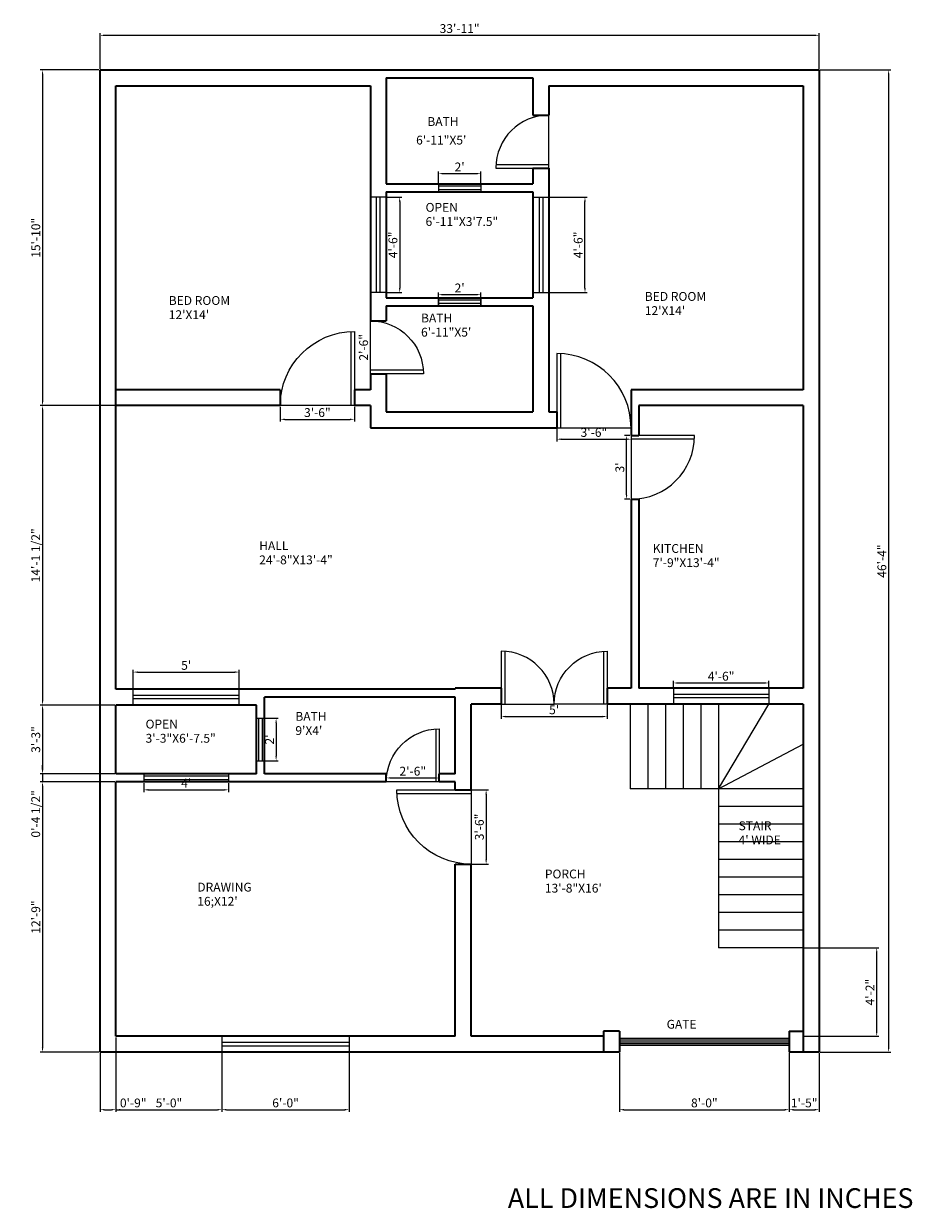
# Model space of a CAD drawing. Units: inches. Extents: x 2169 to 2672, y 1452 to 2123.
import ezdxf

# ---------------------------------------------------------------- set-up
doc = ezdxf.new("R2010")
doc.units = ezdxf.units.IN
for name, color, linetype, lineweight in [('A-ANNO-DIMS', 2, 'Continuous', 18), ('A-ANNO-TEXT', 20, 'Continuous', 18), ('A-AREA-IDEN', 20, 'Continuous', 18), ('A-FLOR-STRS', 200, 'Continuous', 25), ('DOORS', 104, 'Continuous', 25), ('WALL', 200, 'Continuous', 35), ('WINDOWS', 4, 'Continuous', 18)]:
    doc.layers.add(name, color=color, linetype=linetype, lineweight=lineweight)
doc.styles.get("Standard").update_dxf_attribs({"font": 'arial.ttf', "height": 5})
doc.dimstyles.new('ISO-25', dxfattribs={"dimtxt": 5, "dimasz": 2.5, "dimexe": 1.25, "dimexo": 0.625, "dimtad": 1, "dimlunit": 3, "dimtxsty": 'Standard', "dimcen": 2.5, "dimadec": 0, "dimazin": 0, "dimtfac": 1, "dimtmove": 0, "dimatfit": 3, "dimfxl": 1, "dimarcsym": 0})

# ---------------------------------------------------------------- blocks, each defined once
blk = doc.blocks.new('*D1')
at = {"layer": 'A-ANNO-DIMS', "color": 0, "lineweight": -2, "transparency": 16777216}
for p, q in [((2620.28, 2096.79), (2660.2, 2096.79)), ((2658.95, 2094.29), (2658.95, 1543.29)), ((2620.28, 1540.79), (2660.2, 1540.79))]:
    blk.add_line(p, q, dxfattribs=at)
at = {"layer": 'A-ANNO-DIMS', "color": 0, "transparency": 16777216}
for points in [[(2658.53, 2094.29), (2659.36, 2094.29), (2658.95, 2096.79)], [(2658.53, 1543.29), (2659.36, 1543.29), (2658.95, 1540.79)]]:
    blk.add_solid(points, dxfattribs=at)
at = {"layer": 'Defpoints', "color": 0, "transparency": 16777216}
for p in [(2619.65, 2096.79), (2619.65, 1540.79), (2658.95, 1540.79)]:
    blk.add_point(p, dxfattribs=at)
at = {"layer": 'A-ANNO-DIMS', "color": 0, "transparency": 16777216, "insert": (2655.77, 1818.79), "char_height": 5, "attachment_point": 5, "rotation": 90}
blk.add_mtext('46\'-4"', dxfattribs=at)
blk = doc.blocks.new('*D2')
at = {"layer": 'A-ANNO-DIMS', "color": 0, "lineweight": -2, "transparency": 16777216}
for p, q in [((2212.65, 2097.41), (2212.65, 2117.66)), ((2215.15, 2116.41), (2617.15, 2116.41)), ((2619.65, 2097.41), (2619.65, 2117.66))]:
    blk.add_line(p, q, dxfattribs=at)
at = {"layer": 'A-ANNO-DIMS', "color": 0, "transparency": 16777216}
for points in [[(2215.15, 2116.83), (2215.15, 2115.99), (2212.65, 2116.41)], [(2617.15, 2116.83), (2617.15, 2115.99), (2619.65, 2116.41)]]:
    blk.add_solid(points, dxfattribs=at)
at = {"layer": 'Defpoints', "color": 0, "transparency": 16777216}
for p in [(2619.65, 2116.41), (2212.65, 2096.79), (2619.65, 2096.79)]:
    blk.add_point(p, dxfattribs=at)
at = {"layer": 'A-ANNO-DIMS', "color": 0, "transparency": 16777216, "insert": (2416.15, 2119.59), "char_height": 5, "attachment_point": 5}
blk.add_mtext('33\'-11"', dxfattribs=at)
blk = doc.blocks.new('*D3')
at = {"layer": 'A-ANNO-DIMS', "color": 0, "lineweight": -2, "transparency": 16777216}
for p, q in [((2314.65, 1906.16), (2314.65, 1897.78)), ((2356.65, 1906.16), (2356.65, 1897.78)), ((2317.15, 1899.03), (2354.15, 1899.03))]:
    blk.add_line(p, q, dxfattribs=at)
at = {"layer": 'A-ANNO-DIMS', "color": 0, "transparency": 16777216}
for points in [[(2317.15, 1899.45), (2317.15, 1898.62), (2314.65, 1899.03)], [(2354.15, 1899.45), (2354.15, 1898.62), (2356.65, 1899.03)]]:
    blk.add_solid(points, dxfattribs=at)
at = {"layer": 'Defpoints', "color": 0, "transparency": 16777216}
for p in [(2314.65, 1906.79), (2356.65, 1906.79), (2356.65, 1899.03)]:
    blk.add_point(p, dxfattribs=at)
at = {"layer": 'A-ANNO-DIMS', "color": 0, "transparency": 16777216, "insert": (2335.65, 1902.21), "char_height": 5, "attachment_point": 5}
blk.add_mtext('3\'-6"', dxfattribs=at)
blk = doc.blocks.new('*D4')
at = {"layer": 'A-ANNO-DIMS', "color": 0, "lineweight": -2, "transparency": 16777216}
for p, q in [((2365.65, 1927.29), (2365.65, 1952.29)), ((2366.28, 1954.79), (2366.9, 1954.79)), ((2366.28, 1924.79), (2366.9, 1924.79))]:
    blk.add_line(p, q, dxfattribs=at)
at = {"layer": 'A-ANNO-DIMS', "color": 0, "transparency": 16777216}
for points in [[(2365.24, 1952.29), (2366.07, 1952.29), (2365.65, 1954.79)], [(2365.24, 1927.29), (2366.07, 1927.29), (2365.65, 1924.79)]]:
    blk.add_solid(points, dxfattribs=at)
at = {"layer": 'Defpoints', "color": 0, "transparency": 16777216}
for p in [(2365.65, 1954.79), (2365.65, 1954.79), (2365.65, 1924.79)]:
    blk.add_point(p, dxfattribs=at)
at = {"layer": 'A-ANNO-DIMS', "color": 0, "transparency": 16777216, "insert": (2362.48, 1939.79), "char_height": 5, "attachment_point": 5, "rotation": 90}
blk.add_mtext('2\'-6"', dxfattribs=at)
blk = doc.blocks.new('*D5')
at = {"layer": 'A-ANNO-DIMS', "color": 0, "lineweight": -2, "transparency": 16777216}
for p, q in [((2471.15, 1893.66), (2471.15, 1886.54)), ((2513.15, 1893.66), (2513.15, 1886.54)), ((2473.65, 1887.79), (2510.65, 1887.79))]:
    blk.add_line(p, q, dxfattribs=at)
at = {"layer": 'A-ANNO-DIMS', "color": 0, "transparency": 16777216}
for points in [[(2473.65, 1888.21), (2473.65, 1887.37), (2471.15, 1887.79)], [(2510.65, 1888.21), (2510.65, 1887.37), (2513.15, 1887.79)]]:
    blk.add_solid(points, dxfattribs=at)
at = {"layer": 'Defpoints', "color": 0, "transparency": 16777216}
for p in [(2471.15, 1894.29), (2513.15, 1894.29), (2513.15, 1887.79)]:
    blk.add_point(p, dxfattribs=at)
at = {"layer": 'A-ANNO-DIMS', "color": 0, "transparency": 16777216, "insert": (2492.15, 1890.97), "char_height": 5, "attachment_point": 5}
blk.add_mtext('3\'-6"', dxfattribs=at)
blk = doc.blocks.new('*D6')
at = {"layer": 'A-ANNO-DIMS', "color": 0, "lineweight": -2, "transparency": 16777216}
for p, q in [((2512.53, 1889.79), (2509.4, 1889.79)), ((2510.65, 1856.29), (2510.65, 1887.29)), ((2512.53, 1853.79), (2509.4, 1853.79))]:
    blk.add_line(p, q, dxfattribs=at)
at = {"layer": 'A-ANNO-DIMS', "color": 0, "transparency": 16777216}
for points in [[(2510.24, 1887.29), (2511.07, 1887.29), (2510.65, 1889.79)], [(2510.24, 1856.29), (2511.07, 1856.29), (2510.65, 1853.79)]]:
    blk.add_solid(points, dxfattribs=at)
at = {"layer": 'Defpoints', "color": 0, "transparency": 16777216}
for p in [(2510.65, 1889.79), (2513.15, 1889.79), (2513.15, 1853.79)]:
    blk.add_point(p, dxfattribs=at)
at = {"layer": 'A-ANNO-DIMS', "color": 0, "transparency": 16777216, "insert": (2507.47, 1871.79), "char_height": 5, "attachment_point": 5, "rotation": 90}
blk.add_mtext("3'", dxfattribs=at)
blk = doc.blocks.new('*D7')
at = {"layer": 'A-ANNO-DIMS', "color": 0, "lineweight": -2, "transparency": 16777216}
for p, q in [((2439.65, 1737.16), (2439.65, 1729.54)), ((2499.65, 1737.16), (2499.65, 1729.54)), ((2442.15, 1730.79), (2497.15, 1730.79))]:
    blk.add_line(p, q, dxfattribs=at)
at = {"layer": 'A-ANNO-DIMS', "color": 0, "transparency": 16777216}
for points in [[(2442.15, 1731.21), (2442.15, 1730.37), (2439.65, 1730.79)], [(2497.15, 1731.21), (2497.15, 1730.37), (2499.65, 1730.79)]]:
    blk.add_solid(points, dxfattribs=at)
at = {"layer": 'Defpoints', "color": 0, "transparency": 16777216}
for p in [(2439.65, 1737.79), (2499.65, 1737.79), (2499.65, 1730.79)]:
    blk.add_point(p, dxfattribs=at)
at = {"layer": 'A-ANNO-DIMS', "color": 0, "transparency": 16777216, "insert": (2469.65, 1733.96), "char_height": 5, "attachment_point": 5}
blk.add_mtext("5'", dxfattribs=at)
blk = doc.blocks.new('*D8')
at = {"layer": 'A-ANNO-DIMS', "color": 0, "lineweight": -2, "transparency": 16777216}
for p, q in [((2374.65, 1694.54), (2374.65, 1697.29)), ((2404.65, 1694.41), (2404.65, 1697.29)), ((2377.15, 1696.04), (2402.15, 1696.04))]:
    blk.add_line(p, q, dxfattribs=at)
at = {"layer": 'A-ANNO-DIMS', "color": 0, "transparency": 16777216}
for points in [[(2377.15, 1696.46), (2377.15, 1695.62), (2374.65, 1696.04)], [(2402.15, 1696.46), (2402.15, 1695.62), (2404.65, 1696.04)]]:
    blk.add_solid(points, dxfattribs=at)
at = {"layer": 'Defpoints', "color": 0, "transparency": 16777216}
for p in [(2374.65, 1693.92), (2404.65, 1696.04), (2404.65, 1693.79)]:
    blk.add_point(p, dxfattribs=at)
at = {"layer": 'A-ANNO-DIMS', "color": 0, "transparency": 16777216, "insert": (2389.65, 1699.22), "char_height": 5, "attachment_point": 5}
blk.add_mtext('2\'-6"', dxfattribs=at)
blk = doc.blocks.new('*D9')
at = {"layer": 'A-ANNO-DIMS', "color": 0, "lineweight": -2, "transparency": 16777216}
for p, q in [((2423.28, 1689.29), (2432.41, 1689.29)), ((2431.16, 1686.79), (2431.16, 1649.79)), ((2423.28, 1647.29), (2432.41, 1647.29))]:
    blk.add_line(p, q, dxfattribs=at)
at = {"layer": 'A-ANNO-DIMS', "color": 0, "transparency": 16777216}
for points in [[(2430.74, 1686.79), (2431.58, 1686.79), (2431.16, 1689.29)], [(2430.74, 1649.79), (2431.58, 1649.79), (2431.16, 1647.29)]]:
    blk.add_solid(points, dxfattribs=at)
at = {"layer": 'Defpoints', "color": 0, "transparency": 16777216}
for p in [(2422.65, 1689.29), (2422.65, 1647.29), (2431.16, 1647.29)]:
    blk.add_point(p, dxfattribs=at)
at = {"layer": 'A-ANNO-DIMS', "color": 0, "transparency": 16777216, "insert": (2427.98, 1668.29), "char_height": 5, "attachment_point": 5, "rotation": 90}
blk.add_mtext('3\'-6"', dxfattribs=at)
blk = doc.blocks.new('*D10')
at = {"layer": 'A-ANNO-DIMS', "color": 0, "lineweight": -2, "transparency": 16777216}
for p, q in [((2537.15, 1747.41), (2537.15, 1751.04)), ((2591.15, 1747.41), (2591.15, 1751.04)), ((2539.65, 1749.79), (2588.65, 1749.79))]:
    blk.add_line(p, q, dxfattribs=at)
at = {"layer": 'A-ANNO-DIMS', "color": 0, "transparency": 16777216}
for points in [[(2539.65, 1750.2), (2539.65, 1749.37), (2537.15, 1749.79)], [(2588.65, 1750.2), (2588.65, 1749.37), (2591.15, 1749.79)]]:
    blk.add_solid(points, dxfattribs=at)
at = {"layer": 'Defpoints', "color": 0, "transparency": 16777216}
for p in [(2537.15, 1746.79), (2591.15, 1749.79), (2591.15, 1746.79)]:
    blk.add_point(p, dxfattribs=at)
at = {"layer": 'A-ANNO-DIMS', "color": 0, "transparency": 16777216, "insert": (2564.15, 1752.96), "char_height": 5, "attachment_point": 5}
blk.add_mtext('4\'-6"', dxfattribs=at)
blk = doc.blocks.new('*D11')
at = {"layer": 'A-ANNO-DIMS', "color": 0, "lineweight": -2, "transparency": 16777216}
for p, q in [((2231.4, 1746.91), (2231.4, 1757.2)), ((2291.4, 1746.91), (2291.4, 1757.2)), ((2233.9, 1755.95), (2288.9, 1755.95))]:
    blk.add_line(p, q, dxfattribs=at)
at = {"layer": 'A-ANNO-DIMS', "color": 0, "transparency": 16777216}
for points in [[(2233.9, 1756.36), (2233.9, 1755.53), (2231.4, 1755.95)], [(2288.9, 1756.36), (2288.9, 1755.53), (2291.4, 1755.95)]]:
    blk.add_solid(points, dxfattribs=at)
at = {"layer": 'Defpoints', "color": 0, "transparency": 16777216}
for p in [(2291.4, 1755.95), (2231.4, 1746.29), (2291.4, 1746.29)]:
    blk.add_point(p, dxfattribs=at)
at = {"layer": 'A-ANNO-DIMS', "color": 0, "transparency": 16777216, "insert": (2261.4, 1759.11), "char_height": 5, "attachment_point": 5}
blk.add_mtext("5'", dxfattribs=at)
blk = doc.blocks.new('*D12')
at = {"layer": 'A-ANNO-DIMS', "color": 0, "lineweight": -2, "transparency": 16777216}
for p, q in [((2237.4, 1693.16), (2237.4, 1688.06)), ((2285.4, 1693.16), (2285.4, 1688.06)), ((2239.9, 1689.31), (2282.9, 1689.31))]:
    blk.add_line(p, q, dxfattribs=at)
at = {"layer": 'A-ANNO-DIMS', "color": 0, "transparency": 16777216}
for points in [[(2239.9, 1689.73), (2239.9, 1688.89), (2237.4, 1689.31)], [(2282.9, 1689.73), (2282.9, 1688.89), (2285.4, 1689.31)]]:
    blk.add_solid(points, dxfattribs=at)
at = {"layer": 'Defpoints', "color": 0, "transparency": 16777216}
for p in [(2237.4, 1693.79), (2285.4, 1693.79), (2285.4, 1689.31)]:
    blk.add_point(p, dxfattribs=at)
at = {"layer": 'A-ANNO-DIMS', "color": 0, "transparency": 16777216, "insert": (2261.4, 1692.44), "char_height": 5, "attachment_point": 5}
blk.add_mtext("4'", dxfattribs=at)
blk = doc.blocks.new('*D13')
at = {"layer": 'A-ANNO-DIMS', "color": 0, "lineweight": -2, "transparency": 16777216}
for p, q in [((2306.28, 1729.79), (2313.55, 1729.79)), ((2312.3, 1727.29), (2312.3, 1708.29)), ((2306.28, 1705.79), (2313.55, 1705.79))]:
    blk.add_line(p, q, dxfattribs=at)
at = {"layer": 'A-ANNO-DIMS', "color": 0, "transparency": 16777216}
for points in [[(2311.89, 1727.29), (2312.72, 1727.29), (2312.3, 1729.79)], [(2311.89, 1708.29), (2312.72, 1708.29), (2312.3, 1705.79)]]:
    blk.add_solid(points, dxfattribs=at)
at = {"layer": 'Defpoints', "color": 0, "transparency": 16777216}
for p in [(2305.65, 1729.79), (2305.65, 1705.79), (2312.3, 1705.79)]:
    blk.add_point(p, dxfattribs=at)
at = {"layer": 'A-ANNO-DIMS', "color": 0, "transparency": 16777216, "insert": (2309.17, 1717.79), "char_height": 5, "attachment_point": 5, "rotation": 90}
blk.add_mtext("2'", dxfattribs=at)
blk = doc.blocks.new('*D14')
at = {"layer": 'A-ANNO-DIMS', "color": 0, "lineweight": -2, "transparency": 16777216}
for p, q in [((2404.15, 2032.91), (2404.15, 2039.36)), ((2428.15, 2032.91), (2428.15, 2039.36)), ((2406.65, 2038.11), (2425.65, 2038.11))]:
    blk.add_line(p, q, dxfattribs=at)
at = {"layer": 'A-ANNO-DIMS', "color": 0, "transparency": 16777216}
for points in [[(2406.65, 2038.53), (2406.65, 2037.69), (2404.15, 2038.11)], [(2425.65, 2038.53), (2425.65, 2037.69), (2428.15, 2038.11)]]:
    blk.add_solid(points, dxfattribs=at)
at = {"layer": 'Defpoints', "color": 0, "transparency": 16777216}
for p in [(2404.15, 2032.29), (2428.15, 2038.11), (2428.15, 2032.29)]:
    blk.add_point(p, dxfattribs=at)
at = {"layer": 'A-ANNO-DIMS', "color": 0, "transparency": 16777216, "insert": (2416.15, 2041.25), "char_height": 5, "attachment_point": 5}
blk.add_mtext("2'", dxfattribs=at)
blk = doc.blocks.new('*D15')
at = {"layer": 'A-ANNO-DIMS', "color": 0, "lineweight": -2, "transparency": 16777216}
for p, q in [((2375.28, 2024.79), (2383.5, 2024.79)), ((2382.25, 2022.29), (2382.25, 1973.29)), ((2375.28, 1970.79), (2383.5, 1970.79))]:
    blk.add_line(p, q, dxfattribs=at)
at = {"layer": 'A-ANNO-DIMS', "color": 0, "transparency": 16777216}
for points in [[(2381.83, 2022.29), (2382.66, 2022.29), (2382.25, 2024.79)], [(2381.83, 1973.29), (2382.66, 1973.29), (2382.25, 1970.79)]]:
    blk.add_solid(points, dxfattribs=at)
at = {"layer": 'Defpoints', "color": 0, "transparency": 16777216}
for p in [(2374.65, 2024.79), (2374.65, 1970.79), (2382.25, 1970.79)]:
    blk.add_point(p, dxfattribs=at)
at = {"layer": 'A-ANNO-DIMS', "color": 0, "transparency": 16777216, "insert": (2379.07, 1997.79), "char_height": 5, "attachment_point": 5, "rotation": 90}
blk.add_mtext('4\'-6"', dxfattribs=at)
blk = doc.blocks.new('*D16')
at = {"layer": 'A-ANNO-DIMS', "color": 0, "lineweight": -2, "transparency": 16777216}
for p, q in [((2467.28, 2024.79), (2488.36, 2024.79)), ((2487.11, 1973.29), (2487.11, 2022.29)), ((2467.28, 1970.79), (2488.36, 1970.79))]:
    blk.add_line(p, q, dxfattribs=at)
at = {"layer": 'A-ANNO-DIMS', "color": 0, "transparency": 16777216}
for points in [[(2486.69, 2022.29), (2487.52, 2022.29), (2487.11, 2024.79)], [(2486.69, 1973.29), (2487.52, 1973.29), (2487.11, 1970.79)]]:
    blk.add_solid(points, dxfattribs=at)
at = {"layer": 'Defpoints', "color": 0, "transparency": 16777216}
for p in [(2466.65, 2024.79), (2487.11, 2024.79), (2466.65, 1970.79)]:
    blk.add_point(p, dxfattribs=at)
at = {"layer": 'A-ANNO-DIMS', "color": 0, "transparency": 16777216, "insert": (2483.93, 1997.79), "char_height": 5, "attachment_point": 5, "rotation": 90}
blk.add_mtext('4\'-6"', dxfattribs=at)
blk = doc.blocks.new('*D17')
at = {"layer": 'A-ANNO-DIMS', "color": 0, "lineweight": -2, "transparency": 16777216}
for p, q in [((2404.15, 1963.91), (2404.15, 1970.86)), ((2406.65, 1969.61), (2425.65, 1969.61)), ((2428.15, 1963.91), (2428.15, 1970.86))]:
    blk.add_line(p, q, dxfattribs=at)
at = {"layer": 'A-ANNO-DIMS', "color": 0, "transparency": 16777216}
for points in [[(2406.65, 1970.03), (2406.65, 1969.19), (2404.15, 1969.61)], [(2425.65, 1970.03), (2425.65, 1969.19), (2428.15, 1969.61)]]:
    blk.add_solid(points, dxfattribs=at)
at = {"layer": 'Defpoints', "color": 0, "transparency": 16777216}
for p in [(2428.15, 1969.61), (2404.15, 1963.29), (2428.15, 1963.29)]:
    blk.add_point(p, dxfattribs=at)
at = {"layer": 'A-ANNO-DIMS', "color": 0, "transparency": 16777216, "insert": (2416.15, 1972.74), "char_height": 5, "attachment_point": 5}
blk.add_mtext("2'", dxfattribs=at)
blk = doc.blocks.new('DOOR-SWING-30IN')
for p, q in [((0, 30), (0, 0)), ((2, 29.93), (2, 0)), ((0, 0), (30, 0))]:
    blk.add_line(p, q)
blk.add_arc((0, 0), 30, 0, 90)
blk = doc.blocks.new('DOOR-SWING-42IN')
for p, q in [((0, 42), (0, 0)), ((2, 41.95), (2, 0)), ((0, 0), (42, 0))]:
    blk.add_line(p, q)
blk.add_arc((0, 0), 42, 0, 90)
blk = doc.blocks.new('WIN-54IN-9IN-WALL')
for p, q in [((0, 9), (0, 0)), ((0, 9), (54, 9)), ((54, 9), (54, 0)), ((54, 5.5), (0, 5.5)), ((54, 3.5), (0, 3.5)), ((0, 0), (54, 0))]:
    blk.add_line(p, q)
blk = doc.blocks.new('WIN-24IN-4_5IN-WALL')
for p, q in [((0, 24), (4.5, 24)), ((0, 24), (0, 0)), ((1.25, 24), (1.25, 0)), ((3.25, 24), (3.25, 0)), ((4.5, 24), (4.5, 0)), ((0, 0), (4.5, 0))]:
    blk.add_line(p, q)
blk = doc.blocks.new('*D22')
at = {"layer": 'A-ANNO-DIMS', "color": 0, "lineweight": -2, "transparency": 16777216}
for p, q in [((2221.65, 1549.16), (2221.65, 1506.99)), ((2212.65, 1540.16), (2212.65, 1506.99)), ((2215.15, 1508.24), (2219.15, 1508.24)), ((2221.65, 1508.24), (2238.7, 1508.24))]:
    blk.add_line(p, q, dxfattribs=at)
at = {"layer": 'A-ANNO-DIMS', "color": 0, "transparency": 16777216}
for points in [[(2215.15, 1508.66), (2215.15, 1507.82), (2212.65, 1508.24)], [(2219.15, 1508.66), (2219.15, 1507.82), (2221.65, 1508.24)]]:
    blk.add_solid(points, dxfattribs=at)
at = {"layer": 'Defpoints', "color": 0, "transparency": 16777216}
for p in [(2221.65, 1549.79), (2212.65, 1540.79), (2221.65, 1508.24)]:
    blk.add_point(p, dxfattribs=at)
at = {"layer": 'A-ANNO-DIMS', "color": 0, "transparency": 16777216, "insert": (2231.42, 1511.42), "char_height": 5, "attachment_point": 5}
blk.add_mtext('0\'-9"', dxfattribs=at)
blk = doc.blocks.new('*D23')
at = {"layer": 'A-ANNO-DIMS', "color": 0, "lineweight": -2, "transparency": 16777216}
for p, q in [((2221.65, 1549.16), (2221.65, 1506.99)), ((2281.65, 1540.16), (2281.65, 1506.99)), ((2224.15, 1508.24), (2279.15, 1508.24))]:
    blk.add_line(p, q, dxfattribs=at)
at = {"layer": 'A-ANNO-DIMS', "color": 0, "transparency": 16777216}
for points in [[(2224.15, 1508.66), (2224.15, 1507.82), (2221.65, 1508.24)], [(2279.15, 1508.66), (2279.15, 1507.82), (2281.65, 1508.24)]]:
    blk.add_solid(points, dxfattribs=at)
at = {"layer": 'Defpoints', "color": 0, "transparency": 16777216}
for p in [(2221.65, 1549.79), (2281.65, 1540.79), (2281.65, 1508.24)]:
    blk.add_point(p, dxfattribs=at)
at = {"layer": 'A-ANNO-DIMS', "color": 0, "transparency": 16777216, "insert": (2251.65, 1511.42), "char_height": 5, "attachment_point": 5}
blk.add_mtext('5\'-0"', dxfattribs=at)
blk = doc.blocks.new('*D24')
at = {"layer": 'A-ANNO-DIMS', "color": 0, "lineweight": -2, "transparency": 16777216}
for p, q in [((2281.65, 1540.16), (2281.65, 1506.99)), ((2353.65, 1540.16), (2353.65, 1506.99)), ((2284.15, 1508.24), (2351.15, 1508.24))]:
    blk.add_line(p, q, dxfattribs=at)
at = {"layer": 'A-ANNO-DIMS', "color": 0, "transparency": 16777216}
for points in [[(2284.15, 1508.66), (2284.15, 1507.82), (2281.65, 1508.24)], [(2351.15, 1508.66), (2351.15, 1507.82), (2353.65, 1508.24)]]:
    blk.add_solid(points, dxfattribs=at)
at = {"layer": 'Defpoints', "color": 0, "transparency": 16777216}
for p in [(2281.65, 1540.79), (2353.65, 1540.79), (2353.65, 1508.24)]:
    blk.add_point(p, dxfattribs=at)
at = {"layer": 'A-ANNO-DIMS', "color": 0, "transparency": 16777216, "insert": (2317.65, 1511.42), "char_height": 5, "attachment_point": 5}
blk.add_mtext('6\'-0"', dxfattribs=at)
blk = doc.blocks.new('*D25')
at = {"layer": 'A-ANNO-DIMS', "color": 0, "lineweight": -2, "transparency": 16777216}
for p, q in [((2506.65, 1540.16), (2506.65, 1506.99)), ((2602.65, 1540.16), (2602.65, 1506.99)), ((2509.15, 1508.24), (2600.15, 1508.24))]:
    blk.add_line(p, q, dxfattribs=at)
at = {"layer": 'A-ANNO-DIMS', "color": 0, "transparency": 16777216}
for points in [[(2509.15, 1508.66), (2509.15, 1507.82), (2506.65, 1508.24)], [(2600.15, 1508.66), (2600.15, 1507.82), (2602.65, 1508.24)]]:
    blk.add_solid(points, dxfattribs=at)
at = {"layer": 'Defpoints', "color": 0, "transparency": 16777216}
for p in [(2506.65, 1540.79), (2602.65, 1540.79), (2602.65, 1508.24)]:
    blk.add_point(p, dxfattribs=at)
at = {"layer": 'A-ANNO-DIMS', "color": 0, "transparency": 16777216, "insert": (2554.65, 1511.42), "char_height": 5, "attachment_point": 5}
blk.add_mtext('8\'-0"', dxfattribs=at)
blk = doc.blocks.new('*D26')
at = {"layer": 'A-ANNO-DIMS', "color": 0, "lineweight": -2, "transparency": 16777216}
for p, q in [((2602.65, 1540.16), (2602.65, 1506.99)), ((2619.65, 1540.16), (2619.65, 1506.99)), ((2605.15, 1508.24), (2617.15, 1508.24))]:
    blk.add_line(p, q, dxfattribs=at)
at = {"layer": 'A-ANNO-DIMS', "color": 0, "transparency": 16777216}
for points in [[(2605.15, 1508.66), (2605.15, 1507.82), (2602.65, 1508.24)], [(2617.15, 1508.66), (2617.15, 1507.82), (2619.65, 1508.24)]]:
    blk.add_solid(points, dxfattribs=at)
at = {"layer": 'Defpoints', "color": 0, "transparency": 16777216}
for p in [(2602.65, 1540.79), (2619.65, 1540.79), (2619.65, 1508.24)]:
    blk.add_point(p, dxfattribs=at)
at = {"layer": 'A-ANNO-DIMS', "color": 0, "transparency": 16777216, "insert": (2611.15, 1511.42), "char_height": 5, "attachment_point": 5}
blk.add_mtext('1\'-5"', dxfattribs=at)
blk = doc.blocks.new('*D27')
at = {"layer": 'A-ANNO-DIMS', "color": 0, "lineweight": -2, "transparency": 16777216}
for p, q in [((2611.28, 1599.79), (2653.45, 1599.79)), ((2652.2, 1552.29), (2652.2, 1597.29)), ((2611.28, 1549.79), (2653.45, 1549.79))]:
    blk.add_line(p, q, dxfattribs=at)
at = {"layer": 'A-ANNO-DIMS', "color": 0, "transparency": 16777216}
for points in [[(2651.79, 1597.29), (2652.62, 1597.29), (2652.2, 1599.79)], [(2651.79, 1552.29), (2652.62, 1552.29), (2652.2, 1549.79)]]:
    blk.add_solid(points, dxfattribs=at)
at = {"layer": 'Defpoints', "color": 0, "transparency": 16777216}
for p in [(2610.65, 1599.79), (2652.2, 1599.79), (2610.65, 1549.79)]:
    blk.add_point(p, dxfattribs=at)
at = {"layer": 'A-ANNO-DIMS', "color": 0, "transparency": 16777216, "insert": (2649.07, 1574.79), "char_height": 5, "attachment_point": 5, "rotation": 90}
blk.add_mtext('4\'-2"', dxfattribs=at)
blk = doc.blocks.new('*D28')
at = {"layer": 'A-ANNO-DIMS', "color": 0, "lineweight": -2, "transparency": 16777216}
for p, q in [((2212.03, 2096.79), (2178.85, 2096.79)), ((2180.1, 2094.29), (2180.1, 1909.29)), ((2221.03, 1906.79), (2178.85, 1906.79))]:
    blk.add_line(p, q, dxfattribs=at)
at = {"layer": 'A-ANNO-DIMS', "color": 0, "transparency": 16777216}
for points in [[(2179.69, 2094.29), (2180.52, 2094.29), (2180.1, 2096.79)], [(2179.69, 1909.29), (2180.52, 1909.29), (2180.1, 1906.79)]]:
    blk.add_solid(points, dxfattribs=at)
at = {"layer": 'Defpoints', "color": 0, "transparency": 16777216}
for p in [(2212.65, 2096.79), (2180.1, 1906.79), (2221.65, 1906.79)]:
    blk.add_point(p, dxfattribs=at)
at = {"layer": 'A-ANNO-DIMS', "color": 0, "transparency": 16777216, "insert": (2176.93, 2001.79), "char_height": 5, "attachment_point": 5, "rotation": 90}
blk.add_mtext('15\'-10"', dxfattribs=at)
blk = doc.blocks.new('*D29')
at = {"layer": 'A-ANNO-DIMS', "color": 0, "lineweight": -2, "transparency": 16777216}
for p, q in [((2221.03, 1906.79), (2178.85, 1906.79)), ((2180.1, 1904.29), (2180.1, 1739.79)), ((2221.03, 1737.29), (2178.85, 1737.29))]:
    blk.add_line(p, q, dxfattribs=at)
at = {"layer": 'A-ANNO-DIMS', "color": 0, "transparency": 16777216}
for points in [[(2179.69, 1904.29), (2180.52, 1904.29), (2180.1, 1906.79)], [(2179.69, 1739.79), (2180.52, 1739.79), (2180.1, 1737.29)]]:
    blk.add_solid(points, dxfattribs=at)
at = {"layer": 'Defpoints', "color": 0, "transparency": 16777216}
for p in [(2221.65, 1906.79), (2180.1, 1737.29), (2221.65, 1737.29)]:
    blk.add_point(p, dxfattribs=at)
at = {"layer": 'A-ANNO-DIMS', "color": 0, "transparency": 16777216, "insert": (2176.89, 1822.04), "char_height": 5, "attachment_point": 5, "rotation": 90}
blk.add_mtext('14\'-1 1/2"', dxfattribs=at)
blk = doc.blocks.new('*D30')
at = {"layer": 'A-ANNO-DIMS', "color": 0, "lineweight": -2, "transparency": 16777216}
for p, q in [((2221.03, 1737.29), (2178.85, 1737.29)), ((2180.1, 1734.79), (2180.1, 1700.79)), ((2221.03, 1698.29), (2178.85, 1698.29))]:
    blk.add_line(p, q, dxfattribs=at)
at = {"layer": 'A-ANNO-DIMS', "color": 0, "transparency": 16777216}
for points in [[(2179.69, 1734.79), (2180.52, 1734.79), (2180.1, 1737.29)], [(2179.69, 1700.79), (2180.52, 1700.79), (2180.1, 1698.29)]]:
    blk.add_solid(points, dxfattribs=at)
at = {"layer": 'Defpoints', "color": 0, "transparency": 16777216}
for p in [(2221.65, 1737.29), (2180.1, 1698.29), (2221.65, 1698.29)]:
    blk.add_point(p, dxfattribs=at)
at = {"layer": 'A-ANNO-DIMS', "color": 0, "transparency": 16777216, "insert": (2176.92, 1717.79), "char_height": 5, "attachment_point": 5, "rotation": 90}
blk.add_mtext('3\'-3"', dxfattribs=at)
blk = doc.blocks.new('*D31')
at = {"layer": 'A-ANNO-DIMS', "color": 0, "lineweight": -2, "transparency": 16777216}
for p, q in [((2180.1, 1700.79), (2180.1, 1703.29)), ((2221.03, 1698.29), (2178.85, 1698.29)), ((2180.1, 1698.29), (2180.1, 1693.79)), ((2221.03, 1693.79), (2178.85, 1693.79)), ((2180.1, 1691.29), (2180.1, 1662.6))]:
    blk.add_line(p, q, dxfattribs=at)
at = {"layer": 'A-ANNO-DIMS', "color": 0, "transparency": 16777216}
for points in [[(2179.69, 1700.79), (2180.52, 1700.79), (2180.1, 1698.29)], [(2179.69, 1691.29), (2180.52, 1691.29), (2180.1, 1693.79)]]:
    blk.add_solid(points, dxfattribs=at)
at = {"layer": 'Defpoints', "color": 0, "transparency": 16777216}
for p in [(2221.65, 1698.29), (2180.1, 1693.79), (2221.65, 1693.79)]:
    blk.add_point(p, dxfattribs=at)
at = {"layer": 'A-ANNO-DIMS', "color": 0, "transparency": 16777216, "insert": (2176.89, 1675.69), "char_height": 5, "attachment_point": 5, "rotation": 90}
blk.add_mtext('0\'-4 1/2"', dxfattribs=at)
blk = doc.blocks.new('*D32')
at = {"layer": 'A-ANNO-DIMS', "color": 0, "lineweight": -2, "transparency": 16777216}
for p, q in [((2221.03, 1693.79), (2178.85, 1693.79)), ((2180.1, 1691.29), (2180.1, 1543.29)), ((2212.03, 1540.79), (2178.85, 1540.79))]:
    blk.add_line(p, q, dxfattribs=at)
at = {"layer": 'A-ANNO-DIMS', "color": 0, "transparency": 16777216}
for points in [[(2179.69, 1691.29), (2180.52, 1691.29), (2180.1, 1693.79)], [(2179.69, 1543.29), (2180.52, 1543.29), (2180.1, 1540.79)]]:
    blk.add_solid(points, dxfattribs=at)
at = {"layer": 'Defpoints', "color": 0, "transparency": 16777216}
for p in [(2221.65, 1693.79), (2180.1, 1540.79), (2212.65, 1540.79)]:
    blk.add_point(p, dxfattribs=at)
at = {"layer": 'A-ANNO-DIMS', "color": 0, "transparency": 16777216, "insert": (2176.93, 1617.29), "char_height": 5, "attachment_point": 5, "rotation": 90}
blk.add_mtext('12\'-9"', dxfattribs=at)

msp = doc.modelspace()

# ---------------------------------------------------------------- linework, layer by layer
at = {"layer": 'A-FLOR-STRS'}
for p, q in [((2512.654, 1737.789), (2512.654, 1689.789)), ((2522.654, 1737.789), (2522.654, 1689.789)), ((2532.654, 1737.789), (2532.654, 1689.789)), ((2542.654, 1737.789), (2542.654, 1689.789)), ((2552.654, 1737.789), (2552.654, 1689.789)), ((2562.654, 1737.789), (2562.654, 1599.789)), ((2562.654, 1689.789), (2591.154, 1737.789)), ((2562.654, 1689.789), (2610.654, 1715.216)), ((2610.654, 1689.789), (2512.654, 1689.789)), ((2610.654, 1679.789), (2562.654, 1679.789)), ((2610.654, 1669.789), (2562.654, 1669.789)), ((2610.654, 1659.789), (2562.654, 1659.789)), ((2610.654, 1649.789), (2562.654, 1649.789)), ((2610.654, 1639.789), (2562.654, 1639.789)), ((2610.654, 1629.789), (2562.654, 1629.789)), ((2610.654, 1619.789), (2562.654, 1619.789)), ((2610.654, 1609.789), (2562.654, 1609.789)), ((2610.654, 1599.789), (2562.654, 1599.789))]:
    msp.add_line(p, q, dxfattribs=at)
at = {"layer": 'DOORS'}
for p, q in [((2549.154, 1889.789), (2513.154, 1889.789)), ((2513.154, 1889.789), (2513.154, 1853.789)), ((2549.098, 1887.789), (2513.154, 1887.789)), ((2506.654, 1548.708), (2602.654, 1548.708)), ((2506.654, 1547.708), (2602.654, 1547.708)), ((2506.654, 1546.708), (2602.654, 1546.708)), ((2506.654, 1545.708), (2602.654, 1545.708)), ((2506.654, 1544.708), (2602.654, 1544.708))]:
    msp.add_line(p, q, dxfattribs=at)
msp.add_arc((2513.154, 1889.789), 36, 270, 0, dxfattribs=at)
at = {"layer": 'WALL'}
for p, q in [((2212.654, 2096.789), (2619.654, 2096.789)), ((2212.654, 1540.789), (2212.654, 2096.789)), ((2374.654, 2092.289), (2374.654, 2032.289)), ((2374.654, 2092.289), (2457.654, 2092.289)), ((2457.654, 2092.289), (2457.654, 2071.289)), ((2619.654, 2096.789), (2619.654, 1540.789)), ((2221.654, 2087.789), (2365.654, 2087.789)), ((2221.654, 1746.289), (2221.654, 2087.789)), ((2365.654, 2087.789), (2365.654, 1954.789)), ((2466.654, 2087.789), (2466.654, 2071.289)), ((2466.654, 2087.789), (2610.654, 2087.789)), ((2610.654, 2087.789), (2610.654, 1915.789)), ((2457.654, 2071.289), (2466.654, 2071.289)), ((2457.654, 2041.289), (2466.654, 2041.289)), ((2457.654, 2041.289), (2457.654, 2032.289)), ((2466.654, 2041.289), (2466.654, 1903.289)), ((2374.654, 2032.289), (2457.654, 2032.289)), ((2374.654, 2027.789), (2457.654, 2027.789)), ((2374.654, 2027.789), (2374.654, 1967.789)), ((2457.654, 2027.789), (2457.654, 1967.789)), ((2374.654, 1967.789), (2457.654, 1967.789)), ((2374.654, 1963.289), (2457.654, 1963.289)), ((2374.654, 1963.289), (2374.654, 1954.789)), ((2457.654, 1963.289), (2457.654, 1903.289)), ((2365.654, 1954.789), (2374.654, 1954.789)), ((2365.654, 1924.789), (2374.654, 1924.789)), ((2365.654, 1924.789), (2365.654, 1915.789)), ((2374.654, 1924.789), (2374.654, 1903.289)), ((2314.654, 1915.789), (2221.654, 1915.789)), ((2314.654, 1915.789), (2314.654, 1906.789)), ((2365.654, 1915.789), (2356.654, 1915.789)), ((2356.654, 1915.789), (2356.654, 1906.789)), ((2610.654, 1915.789), (2513.154, 1915.789)), ((2513.154, 1915.789), (2513.154, 1889.789)), ((2314.654, 1906.789), (2221.654, 1906.789)), ((2365.654, 1906.789), (2356.654, 1906.789)), ((2365.654, 1906.789), (2365.654, 1894.289)), ((2610.654, 1906.789), (2517.654, 1906.789)), ((2517.654, 1906.789), (2517.654, 1889.789)), ((2610.654, 1906.789), (2610.654, 1746.789)), ((2374.654, 1903.289), (2457.654, 1903.289)), ((2466.654, 1903.289), (2471.154, 1903.289)), ((2471.154, 1903.289), (2471.154, 1894.289)), ((2365.654, 1894.289), (2471.154, 1894.289)), ((2513.154, 1889.789), (2517.654, 1889.789)), ((2513.154, 1853.789), (2517.654, 1853.789)), ((2513.154, 1853.789), (2513.154, 1746.789)), ((2517.654, 1853.789), (2517.654, 1746.789)), ((2413.607, 1746.289), (2221.654, 1746.289)), ((2413.607, 1746.289), (2221.654, 1746.289)), ((2413.607, 1746.289), (2413.607, 1746.789)), ((2439.654, 1746.789), (2413.607, 1746.789)), ((2439.654, 1746.789), (2439.654, 1737.789)), ((2513.154, 1746.789), (2499.654, 1746.789)), ((2499.654, 1746.789), (2499.654, 1737.789)), ((2610.654, 1746.789), (2517.654, 1746.789)), ((2301.154, 1737.289), (2221.654, 1737.289)), ((2221.654, 1698.289), (2221.654, 1737.289)), ((2301.154, 1698.289), (2301.154, 1737.289)), ((2413.607, 1741.789), (2305.654, 1741.789)), ((2305.654, 1698.289), (2305.654, 1741.789)), ((2413.607, 1698.289), (2413.607, 1741.789)), ((2439.654, 1737.789), (2422.654, 1737.789)), ((2422.654, 1689.289), (2422.654, 1737.789)), ((2610.654, 1737.789), (2499.654, 1737.789)), ((2610.654, 1737.789), (2610.654, 1549.789)), ((2301.154, 1698.289), (2221.654, 1698.289)), ((2374.609, 1698.289), (2305.654, 1698.289)), ((2374.656, 1693.789), (2374.609, 1698.289)), ((2413.607, 1698.289), (2404.607, 1698.289)), ((2404.654, 1693.789), (2404.607, 1698.289)), ((2221.654, 1549.789), (2221.654, 1693.789)), ((2374.656, 1693.789), (2221.654, 1693.789)), ((2413.654, 1693.789), (2404.654, 1693.789)), ((2413.654, 1689.289), (2413.654, 1693.789)), ((2413.654, 1689.289), (2422.654, 1689.289)), ((2413.654, 1549.789), (2413.654, 1647.289)), ((2413.654, 1647.289), (2422.654, 1647.289)), ((2422.654, 1549.789), (2422.654, 1647.289)), ((2413.654, 1549.789), (2221.654, 1549.789)), ((2497.654, 1549.789), (2422.654, 1549.789)), ((2497.654, 1552.628), (2497.654, 1540.789)), ((2506.654, 1552.628), (2497.654, 1552.628)), ((2506.654, 1552.628), (2506.654, 1540.789)), ((2602.654, 1552.628), (2602.654, 1540.789)), ((2602.654, 1552.628), (2610.654, 1552.628)), ((2610.654, 1549.789), (2610.654, 1540.789)), ((2506.654, 1540.789), (2212.654, 1540.789)), ((2619.654, 1540.789), (2602.654, 1540.789))]:
    msp.add_line(p, q, dxfattribs=at)
at = {"layer": 'WINDOWS'}
for p, q in [((2231.404, 1737.289), (2231.404, 1746.289)), ((2291.404, 1737.289), (2291.404, 1746.289)), ((2291.404, 1742.789), (2231.404, 1742.789)), ((2291.404, 1740.789), (2231.404, 1740.789)), ((2237.404, 1698.289), (2237.404, 1693.789)), ((2285.404, 1698.289), (2237.404, 1698.289)), ((2285.404, 1697.039), (2237.404, 1697.039)), ((2285.404, 1698.289), (2285.404, 1693.789)), ((2285.404, 1695.039), (2237.404, 1695.039)), ((2237.404, 1693.789), (2285.404, 1693.789)), ((2281.654, 1549.789), (2281.654, 1540.789)), ((2281.654, 1549.789), (2353.654, 1549.789)), ((2353.654, 1549.789), (2353.654, 1540.789)), ((2353.654, 1546.289), (2281.654, 1546.289)), ((2353.654, 1544.289), (2281.654, 1544.289)), ((2281.654, 1540.789), (2353.654, 1540.789))]:
    msp.add_line(p, q, dxfattribs=at)

# ---------------------------------------------------------------- block references
at = {"layer": 'DOORS', "rotation": 89.99999999999774}
msp.add_blockref('DOOR-SWING-30IN', (2466.654, 2041.289), dxfattribs=at)
at = {"layer": 'DOORS', "extrusion": (0, 0, -1), "zscale": -1}
for name, p, rotation in [('DOOR-SWING-30IN', (-2365.654, 1924.789), 90.00000000000047), ('DOOR-SWING-42IN', (-2422.654, 1689.289), 269.9999999999988)]:
    msp.add_blockref(name, p, dxfattribs=dict(at, rotation=rotation))
for name, p in [('DOOR-SWING-42IN', (-2356.654, 1906.789)), ('DOOR-SWING-30IN', (-2499.654, 1737.789)), ('DOOR-SWING-30IN', (-2404.654, 1693.789))]:
    msp.add_blockref(name, p, dxfattribs=at)
at = {"layer": 'DOORS'}
for name, p in [('DOOR-SWING-42IN', (2471.154, 1894.289)), ('DOOR-SWING-30IN', (2439.654, 1737.789))]:
    msp.add_blockref(name, p, dxfattribs=at)
at = {"layer": 'WINDOWS'}
for name, p, rotation in [('WIN-24IN-4_5IN-WALL', (2404.154, 2032.289), 270.0000000000075), ('WIN-54IN-9IN-WALL', (2365.654, 2024.789), 269.9999999999996), ('WIN-54IN-9IN-WALL', (2466.654, 1970.789), 90.00000000000291), ('WIN-24IN-4_5IN-WALL', (2404.154, 1967.789), 270.0000000000075)]:
    msp.add_blockref(name, p, dxfattribs=dict(at, rotation=rotation))
for name, p in [('WIN-54IN-9IN-WALL', (2537.154, 1737.789)), ('WIN-24IN-4_5IN-WALL', (2301.154, 1705.789))]:
    msp.add_blockref(name, p, dxfattribs=at)

# ---------------------------------------------------------------- texts
at = {"layer": 'A-ANNO-TEXT'}
for s, height, p in [('STAIR', 5, (2574.039, 1666.458)), ("4' WIDE", 5, (2574.039, 1658.426)), ('GATE', 5, (2533.316, 1554.09)), ('ALL DIMENSIONS ARE IN INCHES', 11.17446, (2443.42, 1452.615))]:
    msp.add_text(s, height=height, dxfattribs=at).set_placement(p)
at = {"layer": 'A-AREA-IDEN'}
for s, p in [('BATH', (2397.889, 2065.104)), ('6\'-11"X5\'', (2391.525, 2054.592)), ('OPEN', (2396.869, 2016.521)), ('6\'-11"X3\'7.5"', (2396.869, 2008.489)), ('BED ROOM', (2251.523, 1963.798)), ('BED ROOM', (2520.955, 1966.109)), ("12'X14'", (2251.523, 1955.766)), ('BATH', (2394.319, 1953.889)), ("12'X14'", (2520.955, 1958.077)), ('6\'-11"X5\'', (2394.319, 1945.857)), ('HALL', (2302.719, 1825.006)), ('KITCHEN', (2525.462, 1823.433)), ('24\'-8"X13\'-4"', (2302.719, 1816.974)), ('7\'-9"X13\'-4"', (2525.462, 1815.401)), ('BATH', (2323.188, 1728.374)), ('OPEN', (2238.406, 1724.014)), ("9'X4'", (2323.188, 1720.342)), ('3\'-3"X6\'-7.5"', (2238.406, 1715.982)), ('PORCH', (2464.393, 1639.17)), ('DRAWING', (2267.695, 1631.734)), ('13\'-8"X16\'', (2464.393, 1631.138)), ("16;X12'", (2267.695, 1623.702))]:
    msp.add_text(s, height=5, dxfattribs=at).set_placement(p)

# ---------------------------------------------------------------- dimensions: what is measured, and where the dimension line sits
at = {"layer": 'A-ANNO-DIMS'}
for base, p1, p2, override, picture, middle in [((2619.654, 2116.409), (2212.654, 2096.789), (2619.654, 2096.789), {"dimclrd": 0, "dimclre": 0, "dimclrt": 0}, '*D2', (2416.154, 2119.589)), ((2428.154, 2038.11), (2404.154, 2032.289), (2428.154, 2032.289), {"dimclrd": 0, "dimclre": 0, "dimclrt": 0}, '*D14', (2416.154, 2041.245)), ((2428.154, 1969.609), (2404.154, 1963.289), (2428.154, 1963.289), {"dimclrd": 0, "dimclre": 0, "dimclrt": 0}, '*D17', (2416.154, 1972.744)), ((2356.654, 1899.035), (2314.654, 1906.789), (2356.654, 1906.789), {"dimclrd": 0, "dimclre": 0, "dimclrt": 0}, '*D3', (2335.654, 1902.215)), ((2513.154, 1887.789), (2471.154, 1894.289), (2513.154, 1894.289), {"dimclrd": 0, "dimclre": 0, "dimclrt": 0}, '*D5', (2492.154, 1890.968)), ((2291.404, 1755.946), (2231.404, 1746.289), (2291.404, 1746.289), {"dimclrd": 0, "dimclre": 0, "dimclrt": 0}, '*D11', (2261.404, 1759.113)), ((2591.154, 1749.786), (2537.154, 1746.789), (2591.154, 1746.789), {"dimclrd": 0, "dimclre": 0, "dimclrt": 0}, '*D10', (2564.154, 1752.964)), ((2499.654, 1730.789), (2439.654, 1737.789), (2499.654, 1737.789), {"dimclrd": 0, "dimclre": 0, "dimclrt": 0}, '*D7', (2469.654, 1733.957)), ((2404.654, 1696.039), (2374.655, 1693.919), (2404.654, 1693.789), {"dimclrd": 0, "dimclre": 0, "dimclrt": 0}, '*D8', (2389.655, 1699.217)), ((2285.404, 1689.31), (2237.404, 1693.789), (2285.404, 1693.789), {"dimclrd": 0, "dimclre": 0, "dimclrt": 0}, '*D12', (2261.404, 1692.435)), ((2221.654, 1508.239), (2212.654, 1540.789), (2221.654, 1549.789), {"dimdec": 1, "dimlfac": 1, "dimrnd": 0, "dimzin": 1, "dimdsep": 46, "dimlunit": 4, "dimfrac": 2}, '*D22', (2231.425, 1511.417)), ((2281.654, 1508.239), (2221.654, 1549.789), (2281.654, 1540.789), {"dimdec": 1, "dimlfac": 1, "dimrnd": 0, "dimzin": 1, "dimdsep": 46, "dimlunit": 4, "dimfrac": 2}, '*D23', (2251.654, 1511.417)), ((2353.654, 1508.239), (2281.654, 1540.789), (2353.654, 1540.789), {"dimdec": 1, "dimlfac": 1, "dimrnd": 0, "dimzin": 1, "dimdsep": 46, "dimlunit": 4, "dimfrac": 2}, '*D24', (2317.654, 1511.417)), ((2602.654, 1508.239), (2506.654, 1540.789), (2602.654, 1540.789), {"dimdec": 1, "dimlfac": 1, "dimrnd": 0, "dimzin": 1, "dimdsep": 46, "dimlunit": 4, "dimfrac": 2}, '*D25', (2554.654, 1511.417)), ((2619.654, 1508.239), (2602.654, 1540.789), (2619.654, 1540.789), {"dimdec": 1, "dimlfac": 1, "dimrnd": 0, "dimzin": 1, "dimdsep": 46, "dimlunit": 4, "dimfrac": 2}, '*D26', (2611.154, 1511.417))]:
    dim = msp.add_linear_dim(base=base, p1=p1, p2=p2, dimstyle='ISO-25', override=override, dxfattribs=at)
    dim.commit()
    dim.dimension.update_dxf_attribs({"geometry": picture, "text_midpoint": middle})
for base, p1, p2, override, picture, middle in [((2180.104, 1906.789), (2212.654, 2096.789), (2221.654, 1906.789), {"dimdec": 1, "dimlfac": 1, "dimrnd": 0, "dimzin": 1, "dimdsep": 46, "dimlunit": 4, "dimfrac": 2}, '*D28', (2176.926, 2001.789)), ((2658.946, 1540.789), (2619.654, 2096.789), (2619.654, 1540.789), {"dimclrd": 0, "dimclre": 0, "dimclrt": 0}, '*D1', (2655.768, 1818.789)), ((2382.246, 1970.789), (2374.654, 2024.789), (2374.654, 1970.789), {"dimclrd": 0, "dimclre": 0, "dimclrt": 0}, '*D15', (2379.068, 1997.789)), ((2487.106, 2024.789), (2466.654, 1970.789), (2466.654, 2024.789), {"dimclrd": 0, "dimclre": 0, "dimclrt": 0}, '*D16', (2483.928, 1997.789)), ((2365.654, 1954.789), (2365.654, 1924.789), (2365.654, 1954.789), {"dimclrd": 0, "dimclre": 0, "dimclrt": 0}, '*D4', (2362.476, 1939.789)), ((2180.104, 1737.289), (2221.654, 1906.789), (2221.654, 1737.289), {"dimdec": 1, "dimlfac": 1, "dimrnd": 0, "dimzin": 1, "dimdsep": 46, "dimlunit": 4, "dimfrac": 2}, '*D29', (2176.894, 1822.039)), ((2510.654, 1889.789), (2513.154, 1853.789), (2513.154, 1889.789), {"dimclrd": 0, "dimclre": 0, "dimclrt": 0}, '*D6', (2507.474, 1871.789)), ((2180.104, 1698.289), (2221.654, 1737.289), (2221.654, 1698.289), {"dimdec": 1, "dimlfac": 1, "dimrnd": 0, "dimzin": 1, "dimdsep": 46, "dimlunit": 4, "dimfrac": 2}, '*D30', (2176.924, 1717.789)), ((2312.302, 1705.789), (2305.654, 1729.789), (2305.654, 1705.789), {"dimclrd": 0, "dimclre": 0, "dimclrt": 0}, '*D13', (2309.167, 1717.789)), ((2180.104, 1693.789), (2221.654, 1698.289), (2221.654, 1693.789), {"dimdec": 1, "dimlfac": 1, "dimrnd": 0, "dimzin": 1, "dimdsep": 46, "dimlunit": 4, "dimfrac": 2}, '*D31', (2176.894, 1675.693)), ((2180.104, 1540.789), (2221.654, 1693.789), (2212.654, 1540.789), {"dimdec": 1, "dimlfac": 1, "dimrnd": 0, "dimzin": 1, "dimdsep": 46, "dimlunit": 4, "dimfrac": 2}, '*D32', (2176.926, 1617.289)), ((2431.159, 1647.289), (2422.654, 1689.289), (2422.654, 1647.289), {"dimclrd": 0, "dimclre": 0, "dimclrt": 0}, '*D9', (2427.98, 1668.289)), ((2652.204, 1599.789), (2610.654, 1549.789), (2610.654, 1599.789), {"dimdec": 1, "dimlfac": 1, "dimrnd": 0, "dimzin": 1, "dimdsep": 46, "dimlunit": 4, "dimfrac": 2}, '*D27', (2649.069, 1574.789))]:
    dim = msp.add_linear_dim(base=base, p1=p1, p2=p2, angle=90, dimstyle='ISO-25', override=override, dxfattribs=at)
    dim.commit()
    dim.dimension.update_dxf_attribs({"geometry": picture, "text_midpoint": middle})

doc.saveas('drawing.dxf')
